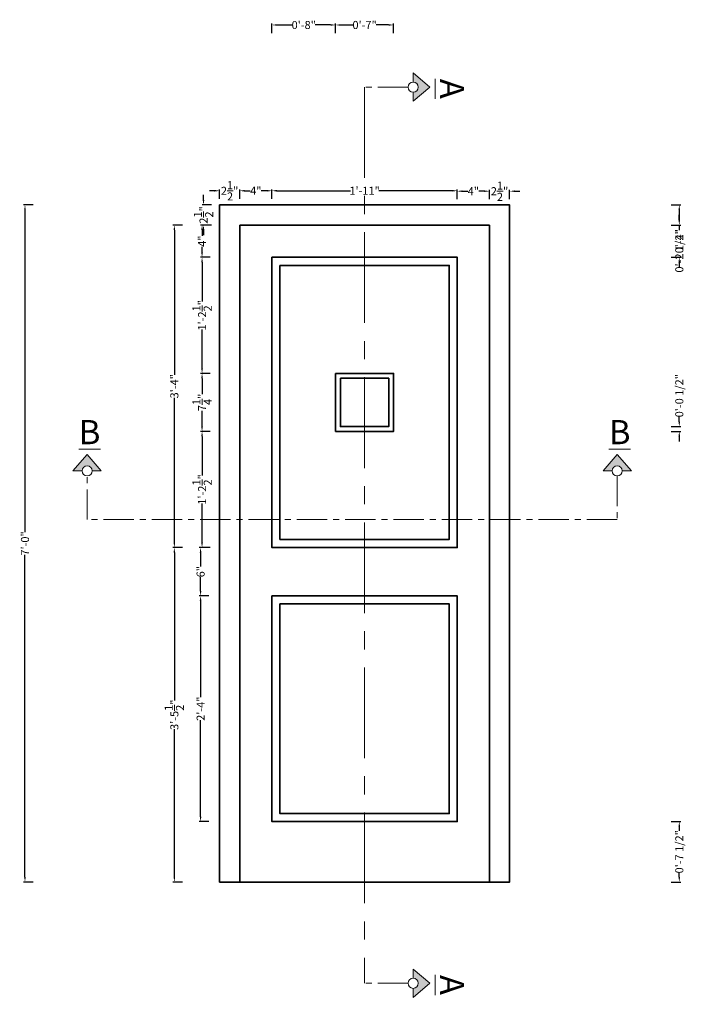
# Model space of a CAD drawing. Units: inches. Extents: x -9 to 130, y -140 to 44.
# Tile 2 of 2: x -9 to 74, y -78 to 44. Entities that reach past the tile are written whole.
import ezdxf

# ---------------------------------------------------------------- set-up
doc = ezdxf.new("R2010")
doc.units = ezdxf.units.IN
doc.header["$LTSCALE"] = 3
doc.header["$MEASUREMENT"] = 0
doc.linetypes.add('CENTER', pattern=[2, 1.25, -0.25, 0.25, -0.25])
for name, color, linetype, lineweight in [('A-ANNO-DIMS', 2, 'Continuous', 18), ('A-ANNO-SYMB', 7, 'Continuous', 18), ('A-ANNO-TEXT', 3, 'Continuous', 18), ('A-DOOR', 4, 'Continuous', 35), ('A-SECT-CUTL', 1, 'CENTER', 18)]:
    doc.layers.add(name, color=color, linetype=linetype, lineweight=lineweight)
doc.styles.get("Standard").update_dxf_attribs({"font": 'arial.ttf'})
doc.dimstyles.get("Standard").update_dxf_attribs({"dimtxt": 1, "dimasz": 0.625, "dimexe": 0.18, "dimexo": 0.0625, "dimgap": 0.09, "dimtad": 0, "dimzin": 0, "dimdsep": 46, "dimlunit": 4, "dimtxsty": 'Standard', "dimcen": 0.09, "dimadec": 0, "dimazin": 0, "dimtfac": 1, "dimtofl": 0, "dimtmove": 0, "dimatfit": 3, "dimfxl": 1, "dimfxlon": 1, "dimtolj": 1, "dimtzin": 0, "dimarcsym": 0})

# ---------------------------------------------------------------- blocks, each defined once
blk = doc.blocks.new('*D1')
at = {"layer": 'A-ANNO-DIMS', "color": 0, "lineweight": -2, "transparency": 16777216}
for p, q in [((15.02, 22.78), (14.4, 22.78)), ((15.65, 21.78), (15.65, 22.96)), ((18.15, 21.78), (18.15, 22.96)), ((18.77, 22.78), (19.4, 22.78))]:
    blk.add_line(p, q, dxfattribs=at)
at = {"layer": 'A-ANNO-DIMS', "color": 0, "transparency": 16777216}
for points in [[(15.02, 22.89), (15.02, 22.68), (15.65, 22.78)], [(18.77, 22.89), (18.77, 22.68), (18.15, 22.78)]]:
    blk.add_solid(points, dxfattribs=at)
at = {"layer": 'Defpoints', "color": 0, "transparency": 16777216}
for p in [(18.15, 22.78), (15.65, 21.03), (18.15, 18.53)]:
    blk.add_point(p, dxfattribs=at)
at = {"layer": 'A-ANNO-DIMS', "color": 0, "transparency": 16777216, "insert": (16.9, 22.78), "char_height": 1, "attachment_point": 5}
blk.add_mtext('\\A1;2{\\H1x;\\S1/2;}"', dxfattribs=at)
blk = doc.blocks.new('*D2')
at = {"layer": 'A-ANNO-DIMS', "color": 0, "lineweight": -2, "transparency": 16777216}
for p, q in [((18.15, 21.78), (18.15, 22.96)), ((18.77, 22.78), (19.46, 22.78)), ((21.52, 22.78), (20.83, 22.78)), ((22.15, 21.78), (22.15, 22.96))]:
    blk.add_line(p, q, dxfattribs=at)
at = {"layer": 'A-ANNO-DIMS', "color": 0, "transparency": 16777216}
for points in [[(18.77, 22.89), (18.77, 22.68), (18.15, 22.78)], [(21.52, 22.89), (21.52, 22.68), (22.15, 22.78)]]:
    blk.add_solid(points, dxfattribs=at)
at = {"layer": 'Defpoints', "color": 0, "transparency": 16777216}
for p in [(22.15, 22.78), (18.15, 18.53), (22.15, 14.53)]:
    blk.add_point(p, dxfattribs=at)
at = {"layer": 'A-ANNO-DIMS', "color": 0, "transparency": 16777216, "insert": (20.15, 22.78), "char_height": 1, "attachment_point": 5}
blk.add_mtext('\\A1;4"', dxfattribs=at)
blk = doc.blocks.new('*D3')
at = {"layer": 'A-ANNO-DIMS', "color": 0, "lineweight": -2, "transparency": 16777216}
for p, q in [((22.15, 21.78), (22.15, 22.96)), ((22.77, 22.78), (31.89, 22.78)), ((44.52, 22.78), (35.41, 22.78)), ((45.15, 21.78), (45.15, 22.96))]:
    blk.add_line(p, q, dxfattribs=at)
at = {"layer": 'A-ANNO-DIMS', "color": 0, "transparency": 16777216}
for points in [[(22.77, 22.89), (22.77, 22.68), (22.15, 22.78)], [(44.52, 22.89), (44.52, 22.68), (45.15, 22.78)]]:
    blk.add_solid(points, dxfattribs=at)
at = {"layer": 'Defpoints', "color": 0, "transparency": 16777216}
for p in [(45.15, 22.78), (22.15, 14.53), (45.15, 14.53)]:
    blk.add_point(p, dxfattribs=at)
at = {"layer": 'A-ANNO-DIMS', "color": 0, "transparency": 16777216, "insert": (33.65, 22.78), "char_height": 1, "attachment_point": 5}
blk.add_mtext('\\A1;1\'-11"', dxfattribs=at)
blk = doc.blocks.new('*D4')
at = {"layer": 'A-ANNO-DIMS', "color": 0, "lineweight": -2, "transparency": 16777216}
for p, q in [((45.15, 21.73), (45.15, 22.91)), ((45.77, 22.73), (46.46, 22.73)), ((48.52, 22.73), (47.83, 22.73)), ((49.15, 21.73), (49.15, 22.91))]:
    blk.add_line(p, q, dxfattribs=at)
at = {"layer": 'A-ANNO-DIMS', "color": 0, "transparency": 16777216}
for points in [[(45.77, 22.83), (45.77, 22.63), (45.15, 22.73)], [(48.52, 22.83), (48.52, 22.63), (49.15, 22.73)]]:
    blk.add_solid(points, dxfattribs=at)
at = {"layer": 'Defpoints', "color": 0, "transparency": 16777216}
for p in [(49.15, 22.73), (49.15, 18.53), (45.15, 14.53)]:
    blk.add_point(p, dxfattribs=at)
at = {"layer": 'A-ANNO-DIMS', "color": 0, "transparency": 16777216, "insert": (47.15, 22.73), "char_height": 1, "attachment_point": 5}
blk.add_mtext('\\A1;4"', dxfattribs=at)
blk = doc.blocks.new('*D5')
at = {"layer": 'A-ANNO-DIMS', "color": 0, "lineweight": -2, "transparency": 16777216}
for p, q in [((48.52, 22.73), (47.9, 22.73)), ((49.15, 21.73), (49.15, 22.91)), ((51.65, 21.73), (51.65, 22.91)), ((52.27, 22.73), (52.9, 22.73))]:
    blk.add_line(p, q, dxfattribs=at)
at = {"layer": 'A-ANNO-DIMS', "color": 0, "transparency": 16777216}
for points in [[(48.52, 22.83), (48.52, 22.63), (49.15, 22.73)], [(52.27, 22.83), (52.27, 22.63), (51.65, 22.73)]]:
    blk.add_solid(points, dxfattribs=at)
at = {"layer": 'Defpoints', "color": 0, "transparency": 16777216}
for p in [(51.65, 22.73), (51.65, 21.03), (49.15, 18.53)]:
    blk.add_point(p, dxfattribs=at)
at = {"layer": 'A-ANNO-DIMS', "color": 0, "transparency": 16777216, "insert": (50.4, 22.73), "char_height": 1, "attachment_point": 5}
blk.add_mtext('\\A1;2{\\H1x;\\S1/2;}"', dxfattribs=at)
blk = doc.blocks.new('*D6')
at = {"layer": 'A-ANNO-DIMS', "color": 0, "lineweight": -2, "transparency": 16777216}
for p, q in [((13.66, 21.65), (13.66, 22.28)), ((14.66, 21.03), (13.48, 21.03)), ((14.66, 18.53), (13.48, 18.53)), ((13.66, 17.9), (13.66, 17.28))]:
    blk.add_line(p, q, dxfattribs=at)
at = {"layer": 'A-ANNO-DIMS', "color": 0, "transparency": 16777216}
for points in [[(13.55, 21.65), (13.76, 21.65), (13.66, 21.03)], [(13.55, 17.9), (13.76, 17.9), (13.66, 18.53)]]:
    blk.add_solid(points, dxfattribs=at)
at = {"layer": 'Defpoints', "color": 0, "transparency": 16777216}
for p in [(13.66, 21.03), (15.65, 21.03), (18.15, 18.53)]:
    blk.add_point(p, dxfattribs=at)
at = {"layer": 'A-ANNO-DIMS', "color": 0, "transparency": 16777216, "insert": (13.66, 19.78), "char_height": 1, "attachment_point": 5, "rotation": 90}
blk.add_mtext('\\A1;2{\\H1x;\\S1/2;}"', dxfattribs=at)
blk = doc.blocks.new('*D7')
at = {"layer": 'A-ANNO-DIMS', "color": 0, "lineweight": -2, "transparency": 16777216}
for p, q in [((14.48, 18.53), (13.3, 18.53)), ((13.48, 17.9), (13.48, 17.21)), ((13.48, 15.15), (13.48, 15.84)), ((14.48, 14.53), (13.3, 14.53))]:
    blk.add_line(p, q, dxfattribs=at)
at = {"layer": 'A-ANNO-DIMS', "color": 0, "transparency": 16777216}
for points in [[(13.37, 17.9), (13.58, 17.9), (13.48, 18.53)], [(13.37, 15.15), (13.58, 15.15), (13.48, 14.53)]]:
    blk.add_solid(points, dxfattribs=at)
at = {"layer": 'Defpoints', "color": 0, "transparency": 16777216}
for p in [(13.48, 18.53), (18.15, 18.53), (22.15, 14.53)]:
    blk.add_point(p, dxfattribs=at)
at = {"layer": 'A-ANNO-DIMS', "color": 0, "transparency": 16777216, "insert": (13.48, 16.53), "char_height": 1, "attachment_point": 5, "rotation": 90}
blk.add_mtext('\\A1;4"', dxfattribs=at)
blk = doc.blocks.new('*D8')
at = {"layer": 'A-ANNO-DIMS', "color": 0, "lineweight": -2, "transparency": 16777216}
for p, q in [((14.48, 14.53), (13.3, 14.53)), ((13.48, 13.9), (13.48, 9.06)), ((13.48, 0.75), (13.48, 5.59)), ((14.48, 0.13), (13.3, 0.13))]:
    blk.add_line(p, q, dxfattribs=at)
at = {"layer": 'A-ANNO-DIMS', "color": 0, "transparency": 16777216}
for points in [[(13.37, 13.9), (13.58, 13.9), (13.48, 14.53)], [(13.37, 0.75), (13.58, 0.75), (13.48, 0.13)]]:
    blk.add_solid(points, dxfattribs=at)
at = {"layer": 'Defpoints', "color": 0, "transparency": 16777216}
for p in [(13.48, 14.53), (22.15, 14.53), (30.05, 0.13)]:
    blk.add_point(p, dxfattribs=at)
at = {"layer": 'A-ANNO-DIMS', "color": 0, "transparency": 16777216, "insert": (13.48, 7.33), "char_height": 1, "attachment_point": 5, "rotation": 90}
blk.add_mtext('\\A1;1\'-2{\\H1x;\\S1/2;}"', dxfattribs=at)
blk = doc.blocks.new('*D9')
at = {"layer": 'A-ANNO-DIMS', "color": 0, "lineweight": -2, "transparency": 16777216}
for p, q in [((14.48, 0.13), (13.3, 0.13)), ((13.48, -0.5), (13.48, -2.43)), ((13.48, -6.45), (13.48, -4.51)), ((14.48, -7.07), (13.3, -7.07))]:
    blk.add_line(p, q, dxfattribs=at)
at = {"layer": 'A-ANNO-DIMS', "color": 0, "transparency": 16777216}
for points in [[(13.37, -0.5), (13.58, -0.5), (13.48, 0.13)], [(13.37, -6.45), (13.58, -6.45), (13.48, -7.07)]]:
    blk.add_solid(points, dxfattribs=at)
at = {"layer": 'Defpoints', "color": 0, "transparency": 16777216}
for p in [(13.48, 0.13), (30.05, 0.13), (30.05, -7.07)]:
    blk.add_point(p, dxfattribs=at)
at = {"layer": 'A-ANNO-DIMS', "color": 0, "transparency": 16777216, "insert": (13.48, -3.47), "char_height": 1, "attachment_point": 5, "rotation": 90}
blk.add_mtext('\\A1;7{\\H1x;\\S1/4;}"', dxfattribs=at)
blk = doc.blocks.new('*D10')
at = {"layer": 'A-ANNO-DIMS', "color": 0, "lineweight": -2, "transparency": 16777216}
for p, q in [((14.48, -7.07), (13.3, -7.07)), ((13.48, -7.7), (13.48, -12.54)), ((13.48, -20.85), (13.48, -16.01)), ((14.48, -21.47), (13.3, -21.47))]:
    blk.add_line(p, q, dxfattribs=at)
at = {"layer": 'A-ANNO-DIMS', "color": 0, "transparency": 16777216}
for points in [[(13.37, -7.7), (13.58, -7.7), (13.48, -7.07)], [(13.37, -20.85), (13.58, -20.85), (13.48, -21.47)]]:
    blk.add_solid(points, dxfattribs=at)
at = {"layer": 'Defpoints', "color": 0, "transparency": 16777216}
for p in [(30.05, -7.07), (13.48, -21.47), (22.15, -21.47)]:
    blk.add_point(p, dxfattribs=at)
at = {"layer": 'A-ANNO-DIMS', "color": 0, "transparency": 16777216, "insert": (13.48, -14.27), "char_height": 1, "attachment_point": 5, "rotation": 90}
blk.add_mtext('\\A1;1\'-2{\\H1x;\\S1/2;}"', dxfattribs=at)
blk = doc.blocks.new('*D11')
at = {"layer": 'A-ANNO-DIMS', "color": 0, "lineweight": -2, "transparency": 16777216}
for p, q in [((14.3, -21.47), (13.12, -21.47)), ((13.3, -22.1), (13.3, -23.81)), ((13.3, -26.85), (13.3, -25.14)), ((14.3, -27.47), (13.12, -27.47))]:
    blk.add_line(p, q, dxfattribs=at)
at = {"layer": 'A-ANNO-DIMS', "color": 0, "transparency": 16777216}
for points in [[(13.19, -22.1), (13.4, -22.1), (13.3, -21.47)], [(13.19, -26.85), (13.4, -26.85), (13.3, -27.47)]]:
    blk.add_solid(points, dxfattribs=at)
at = {"layer": 'Defpoints', "color": 0, "transparency": 16777216}
for p in [(22.15, -21.47), (13.3, -27.47), (22.15, -27.47)]:
    blk.add_point(p, dxfattribs=at)
at = {"layer": 'A-ANNO-DIMS', "color": 0, "transparency": 16777216, "insert": (13.3, -24.47), "char_height": 1, "attachment_point": 5, "rotation": 90}
blk.add_mtext('\\A1;6"', dxfattribs=at)
blk = doc.blocks.new('*D12')
at = {"layer": 'A-ANNO-DIMS', "color": 0, "lineweight": -2, "transparency": 16777216}
for p, q in [((14.3, -27.47), (13.12, -27.47)), ((13.3, -28.1), (13.3, -40.05)), ((13.3, -54.85), (13.3, -42.9)), ((14.3, -55.47), (13.12, -55.47))]:
    blk.add_line(p, q, dxfattribs=at)
at = {"layer": 'A-ANNO-DIMS', "color": 0, "transparency": 16777216}
for points in [[(13.19, -28.1), (13.4, -28.1), (13.3, -27.47)], [(13.19, -54.85), (13.4, -54.85), (13.3, -55.47)]]:
    blk.add_solid(points, dxfattribs=at)
at = {"layer": 'Defpoints', "color": 0, "transparency": 16777216}
for p in [(22.15, -27.47), (13.3, -55.47), (22.15, -55.47)]:
    blk.add_point(p, dxfattribs=at)
at = {"layer": 'A-ANNO-DIMS', "color": 0, "transparency": 16777216, "insert": (13.3, -41.47), "char_height": 1, "attachment_point": 5, "rotation": 90}
blk.add_mtext('\\A1;2\'-4"', dxfattribs=at)
blk = doc.blocks.new('*D13')
at = {"layer": 'A-ANNO-DIMS', "color": 0, "lineweight": -2, "transparency": 16777216}
for p, q in [((11.04, -21.47), (9.86, -21.47)), ((10.04, -22.1), (10.04, -40.44)), ((10.04, -62.35), (10.04, -44.01)), ((11.04, -62.97), (9.86, -62.97))]:
    blk.add_line(p, q, dxfattribs=at)
at = {"layer": 'A-ANNO-DIMS', "color": 0, "transparency": 16777216}
for points in [[(9.94, -22.1), (10.14, -22.1), (10.04, -21.47)], [(9.94, -62.35), (10.14, -62.35), (10.04, -62.97)]]:
    blk.add_solid(points, dxfattribs=at)
at = {"layer": 'Defpoints', "color": 0, "transparency": 16777216}
for p in [(10.04, -21.47), (22.15, -21.47), (15.65, -62.97)]:
    blk.add_point(p, dxfattribs=at)
at = {"layer": 'A-ANNO-DIMS', "color": 0, "transparency": 16777216, "insert": (10.04, -42.22), "char_height": 1, "attachment_point": 5, "rotation": 90}
blk.add_mtext('\\A1;3\'-5{\\H1x;\\S1/2;}"', dxfattribs=at)
blk = doc.blocks.new('*D14')
at = {"layer": 'A-ANNO-DIMS', "color": 0, "lineweight": -2, "transparency": 16777216}
for p, q in [((11.04, 18.53), (9.86, 18.53)), ((10.04, 17.9), (10.04, -0.06)), ((10.04, -20.85), (10.04, -2.89)), ((11.04, -21.47), (9.86, -21.47))]:
    blk.add_line(p, q, dxfattribs=at)
at = {"layer": 'A-ANNO-DIMS', "color": 0, "transparency": 16777216}
for points in [[(9.94, 17.9), (10.14, 17.9), (10.04, 18.53)], [(9.94, -20.85), (10.14, -20.85), (10.04, -21.47)]]:
    blk.add_solid(points, dxfattribs=at)
at = {"layer": 'Defpoints', "color": 0, "transparency": 16777216}
for p in [(10.04, 18.53), (23.2, 18.53), (22.15, -21.47)]:
    blk.add_point(p, dxfattribs=at)
at = {"layer": 'A-ANNO-DIMS', "color": 0, "transparency": 16777216, "insert": (10.04, -1.47), "char_height": 1, "attachment_point": 5, "rotation": 90}
blk.add_mtext('\\A1;3\'-4"', dxfattribs=at)
blk = doc.blocks.new('SECTION-MARK')
for p, q in [((0, 0.63), (1.76, 2.68)), ((3.52, 0.63), (1.76, 2.68)), ((1.13, 0.63), (0, 0.63)), ((2.39, 0.63), (3.52, 0.63))]:
    blk.add_line(p, q)
blk.add_circle((1.76, 0.63), 0.628)
blk = doc.blocks.new('*D18')
at = {"layer": 'A-ANNO-DIMS', "color": 0, "lineweight": -2, "ltscale": 3, "transparency": 16777216}
for p, q in [((15.65, -82.24), (15.65, -83.42)), ((51.65, -82.24), (51.65, -83.42)), ((16.27, -83.24), (32.23, -83.24)), ((51.02, -83.24), (35.07, -83.24))]:
    blk.add_line(p, q, dxfattribs=at)
at = {"layer": 'A-ANNO-DIMS', "color": 0, "ltscale": 3, "transparency": 16777216}
for points in [[(16.27, -83.14), (16.27, -83.35), (15.65, -83.24)], [(51.02, -83.14), (51.02, -83.35), (51.65, -83.24)]]:
    blk.add_solid(points, dxfattribs=at)
at = {"layer": 'Defpoints', "color": 0, "ltscale": 3, "transparency": 16777216}
for p in [(15.65, -62.97), (51.65, -62.97), (51.65, -83.24)]:
    blk.add_point(p, dxfattribs=at)
at = {"layer": 'A-ANNO-DIMS', "color": 0, "ltscale": 3, "transparency": 16777216, "insert": (33.65, -83.24), "char_height": 1, "attachment_point": 5}
blk.add_mtext('\\A1;3\'-0"', dxfattribs=at)
blk = doc.blocks.new('*D19')
at = {"layer": 'A-ANNO-DIMS', "color": 0, "lineweight": -2, "ltscale": 3, "transparency": 16777216}
for p, q in [((-7.5, 21.03), (-8.68, 21.03)), ((-8.5, 20.4), (-8.5, -19.56)), ((-8.5, -62.35), (-8.5, -22.39)), ((-7.5, -62.97), (-8.68, -62.97))]:
    blk.add_line(p, q, dxfattribs=at)
at = {"layer": 'A-ANNO-DIMS', "color": 0, "ltscale": 3, "transparency": 16777216}
for points in [[(-8.6, 20.4), (-8.4, 20.4), (-8.5, 21.03)], [(-8.6, -62.35), (-8.4, -62.35), (-8.5, -62.97)]]:
    blk.add_solid(points, dxfattribs=at)
at = {"layer": 'Defpoints', "color": 0, "ltscale": 3, "transparency": 16777216}
for p in [(15.65, 21.03), (-8.5, -62.97), (15.65, -62.97)]:
    blk.add_point(p, dxfattribs=at)
at = {"layer": 'A-ANNO-DIMS', "color": 0, "ltscale": 3, "transparency": 16777216, "insert": (-8.5, -20.97), "char_height": 1, "attachment_point": 5, "rotation": 90}
blk.add_mtext('\\A1;7\'-0"', dxfattribs=at)
blk = doc.blocks.new('*D20')
at = {"layer": 'A-ANNO-DIMS', "color": 0, "lineweight": -2, "ltscale": 3, "transparency": 16777216}
for p, q in [((71.71, 21.03), (72.89, 21.03)), ((72.71, 20.4), (72.71, 19.15)), ((71.71, 18.53), (72.89, 18.53)), ((72.71, 18.53), (72.71, 17.9))]:
    blk.add_line(p, q, dxfattribs=at)
at = {"layer": 'A-ANNO-DIMS', "color": 0, "ltscale": 3, "transparency": 16777216}
for points in [[(72.6, 20.4), (72.81, 20.4), (72.71, 21.03)], [(72.6, 19.15), (72.81, 19.15), (72.71, 18.53)]]:
    blk.add_solid(points, dxfattribs=at)
at = {"layer": 'Defpoints', "color": 0, "ltscale": 3, "transparency": 16777216}
for p in [(51.65, 21.03), (49.15, 18.53), (72.71, 18.53)]:
    blk.add_point(p, dxfattribs=at)
at = {"layer": 'A-ANNO-DIMS', "color": 0, "ltscale": 3, "transparency": 16777216, "insert": (72.71, 15.32), "char_height": 1, "attachment_point": 5, "rotation": 90}
blk.add_mtext('\\A1;0\'-2 1/2"', dxfattribs=at)
blk = doc.blocks.new('*D21')
at = {"layer": 'A-ANNO-DIMS', "color": 0, "lineweight": -2, "ltscale": 3, "transparency": 16777216}
for p, q in [((72.71, 19.15), (72.71, 19.78)), ((71.71, 18.53), (72.89, 18.53)), ((71.71, 14.53), (72.89, 14.53)), ((72.71, 13.9), (72.71, 13.28))]:
    blk.add_line(p, q, dxfattribs=at)
at = {"layer": 'A-ANNO-DIMS', "color": 0, "ltscale": 3, "transparency": 16777216}
for points in [[(72.6, 19.15), (72.81, 19.15), (72.71, 18.53)], [(72.6, 13.9), (72.81, 13.9), (72.71, 14.53)]]:
    blk.add_solid(points, dxfattribs=at)
at = {"layer": 'Defpoints', "color": 0, "ltscale": 3, "transparency": 16777216}
for p in [(49.15, 18.53), (45.15, 14.53), (72.71, 14.53)]:
    blk.add_point(p, dxfattribs=at)
at = {"layer": 'A-ANNO-DIMS', "color": 0, "ltscale": 3, "transparency": 16777216, "insert": (72.71, 16.53), "char_height": 1, "attachment_point": 5, "rotation": 90}
blk.add_mtext('\\A1;0\'-4"', dxfattribs=at)
blk = doc.blocks.new('*D22')
at = {"layer": 'A-ANNO-DIMS', "color": 0, "lineweight": -2, "ltscale": 3, "transparency": 16777216}
for p, q in [((71.71, -55.47), (72.89, -55.47)), ((72.71, -56.1), (72.71, -56.64)), ((72.71, -62.35), (72.71, -61.81)), ((71.71, -62.97), (72.89, -62.97))]:
    blk.add_line(p, q, dxfattribs=at)
at = {"layer": 'A-ANNO-DIMS', "color": 0, "ltscale": 3, "transparency": 16777216}
for points in [[(72.6, -56.1), (72.81, -56.1), (72.71, -55.47)], [(72.6, -62.35), (72.81, -62.35), (72.71, -62.97)]]:
    blk.add_solid(points, dxfattribs=at)
at = {"layer": 'Defpoints', "color": 0, "ltscale": 3, "transparency": 16777216}
for p in [(45.15, -55.47), (49.15, -62.97), (72.71, -62.97)]:
    blk.add_point(p, dxfattribs=at)
at = {"layer": 'A-ANNO-DIMS', "color": 0, "ltscale": 3, "transparency": 16777216, "insert": (72.71, -59.22), "char_height": 1, "attachment_point": 5, "rotation": 90}
blk.add_mtext('\\A1;0\'-7 1/2"', dxfattribs=at)
blk = doc.blocks.new('*D23')
at = {"layer": 'A-ANNO-DIMS', "color": 0, "lineweight": -2, "ltscale": 3, "transparency": 16777216}
for p, q in [((44.15, -82.24), (44.15, -83.42)), ((45.15, -82.24), (45.15, -83.42)), ((43.52, -83.24), (42.9, -83.24)), ((45.77, -83.24), (46.4, -83.24))]:
    blk.add_line(p, q, dxfattribs=at)
at = {"layer": 'A-ANNO-DIMS', "color": 0, "ltscale": 3, "transparency": 16777216}
for points in [[(43.52, -83.14), (43.52, -83.35), (44.15, -83.24)], [(45.77, -83.14), (45.77, -83.35), (45.15, -83.24)]]:
    blk.add_solid(points, dxfattribs=at)
at = {"layer": 'Defpoints', "color": 0, "ltscale": 3, "transparency": 16777216}
for p in [(44.15, -54.47), (45.15, -55.47), (44.15, -83.24)]:
    blk.add_point(p, dxfattribs=at)
at = {"layer": 'A-ANNO-DIMS', "color": 0, "ltscale": 3, "transparency": 16777216, "insert": (41.48, -83.24), "char_height": 1, "attachment_point": 5}
blk.add_mtext('\\A1;0\'-1"', dxfattribs=at)
blk = doc.blocks.new('*D24')
at = {"layer": 'A-ANNO-DIMS', "color": 0, "lineweight": -2, "ltscale": 3, "transparency": 16777216}
for p, q in [((22.15, 42.35), (22.15, 43.53)), ((22.77, 43.35), (24.68, 43.35)), ((29.42, 43.35), (27.52, 43.35)), ((30.05, 42.35), (30.05, 43.53))]:
    blk.add_line(p, q, dxfattribs=at)
at = {"layer": 'A-ANNO-DIMS', "color": 0, "ltscale": 3, "transparency": 16777216}
for points in [[(22.77, 43.45), (22.77, 43.25), (22.15, 43.35)], [(29.42, 43.45), (29.42, 43.25), (30.05, 43.35)]]:
    blk.add_solid(points, dxfattribs=at)
at = {"layer": 'Defpoints', "color": 0, "ltscale": 3, "transparency": 16777216}
for p in [(30.05, 43.35), (22.15, 14.53), (30.05, 0.13)]:
    blk.add_point(p, dxfattribs=at)
at = {"layer": 'A-ANNO-DIMS', "color": 0, "ltscale": 3, "transparency": 16777216, "insert": (26.1, 43.35), "char_height": 1, "attachment_point": 5}
blk.add_mtext('\\A1;0\'-8"', dxfattribs=at)
blk = doc.blocks.new('*D25')
at = {"layer": 'A-ANNO-DIMS', "color": 0, "lineweight": -2, "ltscale": 3, "transparency": 16777216}
for p, q in [((30.05, 42.35), (30.05, 43.53)), ((30.67, 43.35), (32.23, 43.35)), ((36.62, 43.35), (35.07, 43.35)), ((37.25, 42.35), (37.25, 43.53))]:
    blk.add_line(p, q, dxfattribs=at)
at = {"layer": 'A-ANNO-DIMS', "color": 0, "ltscale": 3, "transparency": 16777216}
for points in [[(30.67, 43.45), (30.67, 43.25), (30.05, 43.35)], [(36.62, 43.45), (36.62, 43.25), (37.25, 43.35)]]:
    blk.add_solid(points, dxfattribs=at)
at = {"layer": 'Defpoints', "color": 0, "ltscale": 3, "transparency": 16777216}
for p in [(37.25, 43.35), (30.05, 0.13), (37.25, 0.13)]:
    blk.add_point(p, dxfattribs=at)
at = {"layer": 'A-ANNO-DIMS', "color": 0, "ltscale": 3, "transparency": 16777216, "insert": (33.65, 43.35), "char_height": 1, "attachment_point": 5}
blk.add_mtext('\\A1;0\'-7"', dxfattribs=at)
blk = doc.blocks.new('*D26')
at = {"layer": 'A-ANNO-DIMS', "color": 0, "lineweight": -2, "ltscale": 3, "transparency": 16777216}
for p, q in [((72.71, -5.85), (72.71, -5.22)), ((71.71, -6.47), (72.89, -6.47)), ((71.71, -7.07), (72.89, -7.07)), ((72.71, -7.7), (72.71, -8.32))]:
    blk.add_line(p, q, dxfattribs=at)
at = {"layer": 'A-ANNO-DIMS', "color": 0, "ltscale": 3, "transparency": 16777216}
for points in [[(72.6, -5.85), (72.81, -5.85), (72.71, -6.47)], [(72.6, -7.7), (72.81, -7.7), (72.71, -7.07)]]:
    blk.add_solid(points, dxfattribs=at)
at = {"layer": 'Defpoints', "color": 0, "ltscale": 3, "transparency": 16777216}
for p in [(36.65, -6.47), (37.25, -7.07), (72.71, -6.47)]:
    blk.add_point(p, dxfattribs=at)
at = {"layer": 'A-ANNO-DIMS', "color": 0, "ltscale": 3, "transparency": 16777216, "insert": (72.71, -2.64), "char_height": 1, "attachment_point": 5, "rotation": 90}
blk.add_mtext('\\A1;0\'-0 1/2"', dxfattribs=at)

msp = doc.modelspace()

# ---------------------------------------------------------------- hatches: boundary and pattern name
at = {"layer": 'A-ANNO-SYMB'}
h = msp.add_hatch(color=256, dxfattribs=at)
h.dxf.hatch_style = 1
h.paths.add_polyline_path([(39.68, 37.399), (39.68, 36.269, -0.4142136), (40.308, 35.64, -0.4142136), (39.68, 35.012), (39.68, 33.881), (41.73, 35.64)])
h = msp.add_hatch(color=256, dxfattribs=at)
h.dxf.hatch_style = 1
h.paths.add_polyline_path([(-0.791, -9.925), (-2.55, -11.975), (-1.419, -11.975, -1), (-0.162, -11.975), (0.968, -11.975)])
h = msp.add_hatch(color=256, dxfattribs=at)
h.dxf.hatch_style = 1
h.paths.add_polyline_path([(65, -9.925), (63.241, -11.975), (64.371, -11.975, -1), (65.628, -11.975), (66.759, -11.975)])
h = msp.add_hatch(color=256, dxfattribs=at)
h.dxf.hatch_style = 1
h.paths.add_polyline_path([(39.68, -73.776), (39.68, -74.906, -0.4142136), (40.308, -75.535, -0.4142136), (39.68, -76.163), (39.68, -77.294), (41.73, -75.535)])

# ---------------------------------------------------------------- linework, layer by layer
at = {"layer": 'A-DOOR'}
for p, q in [((18.148, 18.526), (49.148, 18.526)), ((18.148, -62.974), (18.148, 18.526)), ((49.148, 18.526), (49.148, -62.974))]:
    msp.add_line(p, q, dxfattribs=at)
for points in [[(15.648, 21.026), (51.648, 21.026), (51.648, -62.974), (15.648, -62.974)], [(22.148, 14.526), (45.148, 14.526), (45.148, -21.474), (22.148, -21.474)], [(23.148, 13.526), (44.148, 13.526), (44.148, -20.474), (23.148, -20.474)], [(30.048, 0.126), (37.248, 0.126), (37.248, -7.074), (30.048, -7.074)], [(30.648, -0.474), (36.648, -0.474), (36.648, -6.474), (30.648, -6.474)], [(22.148, -27.474), (45.148, -27.474), (45.148, -55.474), (22.148, -55.474)], [(23.148, -28.474), (44.148, -28.474), (44.148, -54.474), (23.148, -54.474)]]:
    msp.add_lwpolyline(points, close=True, dxfattribs=at)
at = {"layer": 'A-SECT-CUTL', "ltscale": 3}
msp.add_line((33.648, 35.64), (33.648, -75.535), dxfattribs=at)
at = {"layer": 'A-SECT-CUTL'}
for p, q in [((39.051, 35.64), (33.648, 35.64)), ((-0.791, -18.007), (-0.791, -12.603)), ((65, -12.603), (65, -18.007)), ((65, -18.007), (-0.791, -18.007)), ((39.051, -75.535), (33.648, -75.535))]:
    msp.add_line(p, q, dxfattribs=at)

# ---------------------------------------------------------------- block references
at = {"layer": 'A-ANNO-SYMB'}
for p, rotation in [((39.051, 37.399), 269.9999999999999), ((39.051, -73.776), 269.9999999999998)]:
    msp.add_blockref('SECTION-MARK', p, dxfattribs=dict(at, rotation=rotation))
for p in [(-2.549, -12.603), (63.241, -12.603)]:
    msp.add_blockref('SECTION-MARK', p, dxfattribs=at)

# ---------------------------------------------------------------- texts
at = {"layer": 'A-ANNO-TEXT', "char_height": 3, "attachment_point": 1, "rotation": 270}
for insert in [(45.999, 36.675), (45.999, -74.5)]:
    msp.add_mtext_dynamic_manual_height_columns('{\\fArial|b1|i0|c0|p34;\\LA}', width=3.20276, gutter_width=1, heights=[0], dxfattribs=dict(at, insert=insert))
at = {"layer": 'A-ANNO-TEXT', "char_height": 3, "attachment_point": 1}
for insert in [(-1.825, -5.656), (63.965, -5.656)]:
    msp.add_mtext_dynamic_manual_height_columns('{\\fArial|b1|i0|c0|p34;\\LB}', width=3.20276, gutter_width=1, heights=[0], dxfattribs=dict(at, insert=insert))

# ---------------------------------------------------------------- dimensions: what is measured, and where the dimension line sits
at = {"layer": 'A-ANNO-DIMS', "ltscale": 3}
for base, p1, p2, picture, middle in [((30.048, 43.349), (22.148, 14.526), (30.048, 0.126), '*D24', (26.098, 43.349)), ((37.248, 43.349), (30.048, 0.126), (37.248, 0.126), '*D25', (33.648, 43.349)), ((44.148, -83.244), (45.148, -55.474), (44.148, -54.474), '*D23', (41.478, -83.244)), ((51.648, -83.244), (15.648, -62.974), (51.648, -62.974), '*D18', (33.648, -83.244))]:
    dim = msp.add_linear_dim(base=base, p1=p1, p2=p2, dimstyle='Standard', override={"dimdec": 1, "dimlfac": 1, "dimrnd": 0, "dimzin": 1, "dimdsep": 46, "dimlunit": 4, "dimfrac": 2}, dxfattribs=at)
    dim.commit()
    dim.dimension.update_dxf_attribs({"geometry": picture, "text_midpoint": middle})
at = {"layer": 'A-ANNO-DIMS'}
for base, p1, p2, picture, middle in [((18.148, 22.781), (15.648, 21.026), (18.148, 18.526), '*D1', (16.898, 22.781)), ((22.148, 22.781), (18.148, 18.526), (22.148, 14.526), '*D2', (20.148, 22.781)), ((45.148, 22.781), (22.148, 14.526), (45.148, 14.526), '*D3', (33.648, 22.781)), ((49.148, 22.729), (45.148, 14.526), (49.148, 18.526), '*D4', (47.148, 22.729)), ((51.648, 22.729), (49.148, 18.526), (51.648, 21.026), '*D5', (50.398, 22.729))]:
    dim = msp.add_linear_dim(base=base, p1=p1, p2=p2, dimstyle='Standard', override={"dimclrd": 0, "dimclre": 0, "dimclrt": 0}, dxfattribs=at)
    dim.commit()
    dim.dimension.update_dxf_attribs({"geometry": picture, "text_midpoint": middle})
for base, p1, p2, picture, middle in [((13.658, 21.026), (18.148, 18.526), (15.648, 21.026), '*D6', (13.658, 19.776)), ((10.04, 18.526), (22.148, -21.474), (23.196, 18.526), '*D14', (10.04, -1.474)), ((13.478, 18.526), (22.148, 14.526), (18.148, 18.526), '*D7', (13.478, 16.526)), ((13.478, 14.526), (30.048, 0.126), (22.148, 14.526), '*D8', (13.478, 7.326)), ((13.478, 0.126), (30.048, -7.074), (30.048, 0.126), '*D9', (13.478, -3.474)), ((13.478, -21.474), (30.048, -7.074), (22.148, -21.474), '*D10', (13.478, -14.274)), ((10.04, -21.474), (15.648, -62.974), (22.148, -21.474), '*D13', (10.04, -42.224)), ((13.298, -27.474), (22.148, -21.474), (22.148, -27.474), '*D11', (13.298, -24.474)), ((13.298, -55.474), (22.148, -27.474), (22.148, -55.474), '*D12', (13.298, -41.474))]:
    dim = msp.add_linear_dim(base=base, p1=p1, p2=p2, angle=90, dimstyle='Standard', override={"dimclrd": 0, "dimclre": 0, "dimclrt": 0}, dxfattribs=at)
    dim.commit()
    dim.dimension.update_dxf_attribs({"geometry": picture, "text_midpoint": middle})
at = {"layer": 'A-ANNO-DIMS', "ltscale": 3}
for base, p1, p2, picture, middle in [((-8.5, -62.974), (15.648, 21.026), (15.648, -62.974), '*D19', (-8.5, -20.974)), ((72.709, 18.526), (51.648, 21.026), (49.148, 18.526), '*D20', (72.709, 15.317)), ((72.709, 14.526), (49.148, 18.526), (45.148, 14.526), '*D21', (72.709, 16.526)), ((72.709, -6.474), (37.248, -7.074), (36.648, -6.474), '*D26', (72.709, -2.64)), ((72.709, -62.974), (45.148, -55.474), (49.148, -62.974), '*D22', (72.709, -59.224))]:
    dim = msp.add_linear_dim(base=base, p1=p1, p2=p2, angle=90, dimstyle='Standard', override={"dimdec": 1, "dimlfac": 1, "dimrnd": 0, "dimzin": 1, "dimdsep": 46, "dimlunit": 4, "dimfrac": 2}, dxfattribs=at)
    dim.commit()
    dim.dimension.update_dxf_attribs({"geometry": picture, "text_midpoint": middle})

doc.saveas('drawing.dxf')
